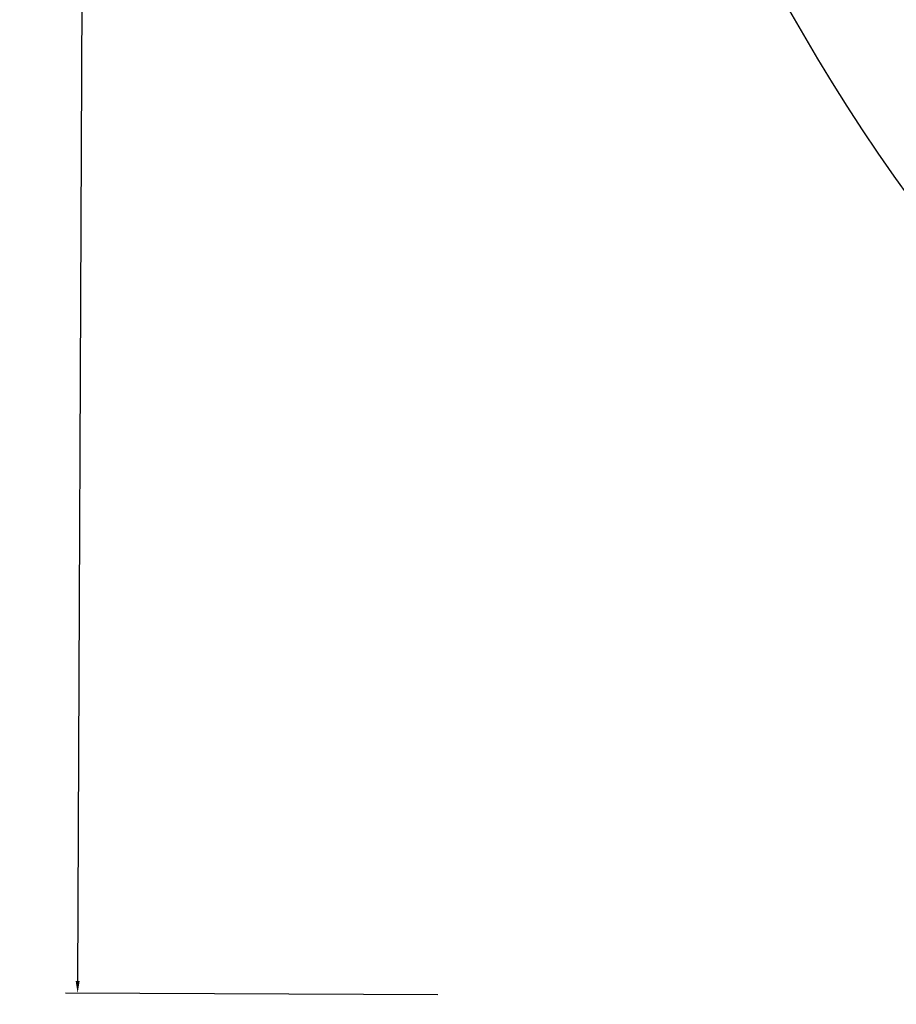
# Model space of a CAD drawing. Units: inches. Extents: x 1901 to 2863, y 888 to 2433.
# Tile 26 of 91: x 2560.41 to 2573.39, y 1361.82 to 1376.41. Entities that reach past the tile are written whole.
import ezdxf

# ---------------------------------------------------------------- set-up
doc = ezdxf.new("R2010")
doc.units = ezdxf.units.IN
doc.layers.add('A-ANNO-DIMS', color=2, linetype='Continuous', lineweight=18)
doc.layers.add('A-DOOR', color=4, linetype='Continuous', lineweight=25)
doc.styles.get("Standard").update_dxf_attribs({"font": 'arial.ttf'})
doc.dimstyles.get("Standard").update_dxf_attribs({"dimtxt": 0.18, "dimasz": 0.18, "dimexe": 0.18, "dimexo": 0.0625, "dimgap": 0.09, "dimtad": 0, "dimtih": 1, "dimtoh": 1, "dimdec": 4, "dimzin": 0, "dimdsep": 46, "dimtxsty": 'Standard', "dimcen": 0.09, "dimadec": 0, "dimazin": 0, "dimtfac": 1, "dimtdec": 4, "dimtofl": 0, "dimtmove": 0, "dimatfit": 3, "dimfxl": 1, "dimtolj": 1, "dimtzin": 0, "dimarcsym": 0})

# ---------------------------------------------------------------- blocks, each defined once
blk = doc.blocks.new('DOOR-29')
blk.add_line((-0.004, -0.016), (-0.004, 35.984))
blk.add_arc((-0.004, 7.119), 28.865, 345.6888, 90)
blk = doc.blocks.new('*D31')
at = {"layer": 'A-ANNO-DIMS', "color": 0, "lineweight": -2, "transparency": 16777216}
for p, q in [((2566.77, 1397.965), (2561.253, 1397.99)), ((2561.432, 1397.81), (2561.35, 1380.173)), ((2561.266, 1362.17), (2561.348, 1379.807)), ((2566.603, 1361.965), (2561.085, 1361.991))]:
    blk.add_line(p, q, dxfattribs=at)
at = {"layer": 'A-ANNO-DIMS', "color": 0, "transparency": 16777216}
for points in [[(2561.402, 1397.81), (2561.462, 1397.809), (2561.433, 1397.99)], [(2561.236, 1362.17), (2561.296, 1362.17), (2561.265, 1361.99)]]:
    blk.add_solid(points, dxfattribs=at)
at = {"layer": 'Defpoints', "color": 0, "transparency": 16777216}
for p in [(2566.833, 1397.964), (2561.265, 1361.99), (2566.665, 1361.965)]:
    blk.add_point(p, dxfattribs=at)
at = {"layer": 'A-ANNO-DIMS', "color": 0, "transparency": 16777216, "insert": (2561.349, 1379.99), "char_height": 0.18, "attachment_point": 5}
blk.add_mtext('\\A1;DOOR D1 36 TYP.', dxfattribs=at)

msp = doc.modelspace()

# ---------------------------------------------------------------- block references
at = {"layer": 'A-DOOR', "rotation": 179.7338121645225}
msp.add_blockref('DOOR-29', (2597.001, 1397.808), dxfattribs=at)

# ---------------------------------------------------------------- dimensions: what is measured, and where the dimension line sits
at = {"layer": 'A-ANNO-DIMS'}
dim = msp.add_linear_dim(base=(2561.265, 1361.99), p1=(2566.833, 1397.964), p2=(2566.665, 1361.965), angle=269.7338, text='DOOR D1 <> TYP.', dimstyle='Standard', override={"dimdec": 0, "dimlfac": 1, "dimrnd": 0, "dimzin": 0, "dimdsep": 46, "dimlunit": 2}, dxfattribs=at)
dim.commit()
dim.dimension.update_dxf_attribs({"geometry": '*D31', "text_midpoint": (2561.349, 1379.99)})

doc.saveas('drawing.dxf')
